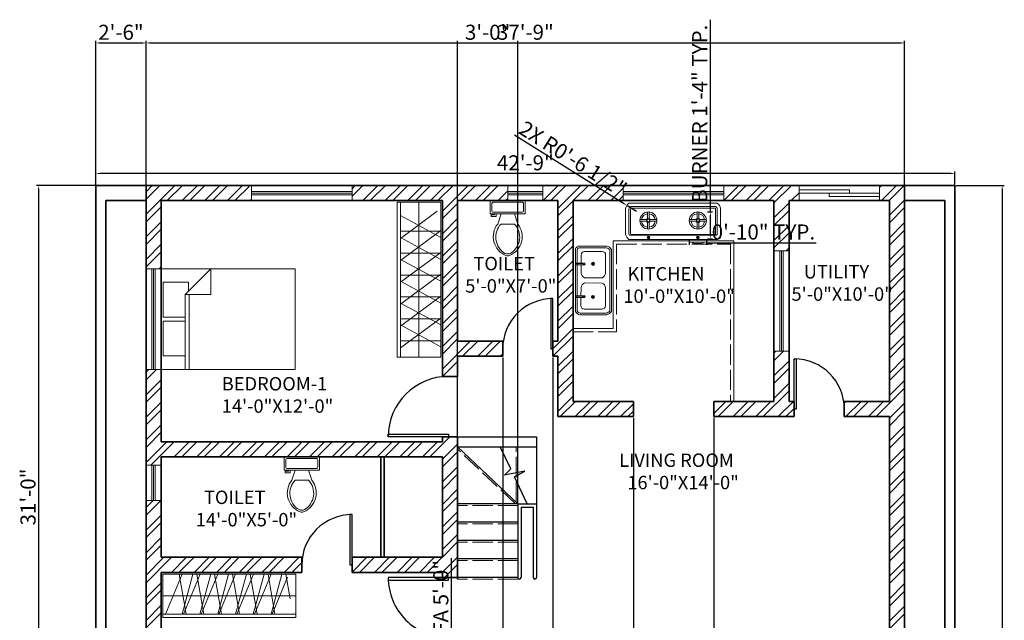
# Model space of a CAD drawing. Units: inches. Extents: x 451 to 1761, y 2292 to 3014.
# Tile 2 of 3: x 451 to 1039, y 2655 to 3014. Entities that reach past the tile are written whole.
import ezdxf

# ---------------------------------------------------------------- set-up
doc = ezdxf.new("R2010")
doc.units = ezdxf.units.IN
doc.linetypes.add('ACAD_ISO02W100', pattern=[15, 12, -3])
for name, color, linetype, lineweight in [('A-ANNO-DIMS', 2, 'Continuous', 18), ('A-AREA-IDEN', 7, 'Continuous', 18), ('A-DOOR', 4, 'Continuous', 25), ('A-EQPM', 8, 'Continuous', 18), ('A-FLOR-CASE', 9, 'Continuous', 18), ('A-FLOR-CASE-HIDN', 9, 'ACAD_ISO02W100', 13), ('A-FLOR-CASE-PATT', 252, 'Continuous', 13), ('A-FLOR-FIXT', 9, 'Continuous', 18), ('A-FLOR-STRS', 7, 'Continuous', 25), ('A-FLOR-STRS-HIDN', 8, 'ACAD_ISO02W100', 13), ('A-FURN', 8, 'Continuous', 18), ('A-GLAZ', 244, 'Continuous', 18), ('A-WALL', 7, 'Continuous', 35), ('A-WALL-PATT', 252, 'Continuous', 13), ('C-PROP', 7, 'Continuous', 35)]:
    doc.layers.add(name, color=color, linetype=linetype, lineweight=lineweight)
doc.styles.get("Standard").update_dxf_attribs({"font": 'arial.ttf'})
doc.dimstyles.new('ISO-25', dxfattribs={"dimtxt": 9, "dimasz": 2.5, "dimexe": 1.25, "dimexo": 0.625, "dimtad": 1, "dimlunit": 3, "dimtxsty": 'Standard', "dimcen": 2.5, "dimadec": 0, "dimazin": 0, "dimtfac": 1, "dimtmove": 0, "dimatfit": 3, "dimfxl": 1, "dimarcsym": 0})

# ---------------------------------------------------------------- blocks, each defined once
blk = doc.blocks.new('*D1')
at = {"layer": 'A-ANNO-DIMS', "color": 0, "lineweight": -2, "transparency": 16777216}
for p, q in [((496.79, 2915.38), (496.79, 2923.19)), ((1009.79, 2915.38), (1009.79, 2923.19)), ((1007.29, 2921.94), (499.29, 2921.94))]:
    blk.add_line(p, q, dxfattribs=at)
at = {"layer": 'A-ANNO-DIMS', "color": 0, "transparency": 16777216}
for points in [[(499.29, 2922.36), (499.29, 2921.52), (496.79, 2921.94)], [(1007.29, 2922.36), (1007.29, 2921.52), (1009.79, 2921.94)]]:
    blk.add_solid(points, dxfattribs=at)
at = {"layer": 'Defpoints', "color": 0, "transparency": 16777216}
for p in [(496.79, 2921.94), (496.79, 2914.76), (1009.79, 2914.76)]:
    blk.add_point(p, dxfattribs=at)
at = {"layer": 'A-ANNO-DIMS', "color": 0, "transparency": 16777216, "insert": (753.29, 2927.16), "char_height": 9, "attachment_point": 5}
blk.add_mtext('42\'-9"', dxfattribs=at)
blk = doc.blocks.new('*U3')
for p, q in [((0, 0), (0, 6)), ((40, 0), (40, 6))]:
    blk.add_line(p, q)
blk.add_lwpolyline([(0, 0), (0, -40), (1.75, -40), (1.75, 0)], close=True)
blk.add_arc((0, 0), 40, 270, 0)
blk = doc.blocks.new('*U4')
for p, q in [((-40, 0), (-40, 6)), ((0, 0), (0, 6))]:
    blk.add_line(p, q)
blk.add_lwpolyline([(0, 0), (0, -40), (-1.75, -40), (-1.75, 0)], close=True)
blk.add_arc((0, 0), 40, 180, 270)
blk = doc.blocks.new('*U5')
for p, q in [((0, 0), (0, 6)), ((40, 0), (40, 6))]:
    blk.add_line(p, q)
blk.add_lwpolyline([(0, 0), (0, -40), (1.75, -40), (1.75, 0)], close=True)
blk.add_arc((0, 0), 40, 270, 0)
blk = doc.blocks.new('Bed - Queen')
for p, q in [((0, -80.00003), (0, 0)), ((0, 0), (59.99999, 0)), ((59.99999, 0), (59.99999, -80.00003)), ((7.99999, -1.2), (28.79998, -1.2)), ((7.99999, -14.4), (7.99999, -1.2)), ((28.79998, -1.2), (28.79998, -14.4)), ((31.19999, -1.2), (51.99999, -1.2)), ((31.19999, -14.4), (31.19999, -1.2)), ((51.99999, -1.2), (51.99999, -16.4)), ((0, -14.4), (44.8, -14.4)), ((44.8, -16.8), (0, -16.8)), ((59.99999, -29.6), (44.8, -14.4)), ((44.8, -14.4), (44.8, -29.6)), ((51.99999, -16.4), (46.79936, -16.4)), ((44.8, -29.6), (59.99999, -29.6)), ((59.99999, -80.00003), (0, -80.00003))]:
    blk.add_line(p, q)
blk = doc.blocks.new('*U10')
for p, q in [((9.5, -6), (9.5, -2)), ((-10, -8.5), (-8, -8.5)), ((-10, -9.5), (-10, -8.5)), ((-7, -9.5), (-10, -9.5)), ((-8, -8.5), (-8, -8)), ((-7, -8), (-7, -9.5)), ((-4, -8), (-6, -14)), ((4, -8), (6, -14)), ((4, -14), (-4, -14))]:
    blk.add_line(p, q)
blk.add_lwpolyline([(10.5, -8), (10.5, 0), (-10.5, 0), (-10.5, -8)], close=True)
for points in [[(-9.5, -2), (-9.5, -6)], [(8.5, -1), (-8.5, -1)], [(-8.5, -7), (8.5, -7)]]:
    blk.add_lwpolyline(points)
for centre, radius, start, end in [((-8.62, -1.88), 0.884, 81.8699, 188.1301), ((8.62, -1.88), 0.884, 351.8699, 98.1301), ((-8.62, -6.12), 0.884, 171.8699, 278.1301), ((8.62, -6.12), 0.884, 261.8699, 8.1301), ((3.52, -21.58), 12.17, 141.46911, 247.97143), ((4.2, -21.82), 11.33, 136.36773, 238.94682), ((-3.52, -21.58), 12.17, 292.02843, 38.53071), ((-4.2, -21.82), 11.33, 301.05301, 43.63209), ((0, -27.88), 4, 245.73182, 294.26817), ((0, -29), 4, 254.86053, 285.13947)]:
    blk.add_arc(centre, radius, start, end)
blk = doc.blocks.new('*D13')
at = {"layer": 'A-ANNO-DIMS', "color": 0, "lineweight": -2, "transparency": 16777216}
for p, q in [((1010.42, 2914.76), (1039.33, 2914.76)), ((1038.08, 2912.26), (1038.08, 2332.26)), ((1010.42, 2329.76), (1039.33, 2329.76))]:
    blk.add_line(p, q, dxfattribs=at)
at = {"layer": 'A-ANNO-DIMS', "color": 0, "transparency": 16777216}
for points in [[(1037.66, 2912.26), (1038.49, 2912.26), (1038.08, 2914.76)], [(1037.66, 2332.26), (1038.49, 2332.26), (1038.08, 2329.76)]]:
    blk.add_solid(points, dxfattribs=at)
at = {"layer": 'Defpoints', "color": 0, "transparency": 16777216}
for p in [(1009.79, 2914.76), (1009.79, 2329.76), (1038.08, 2329.76)]:
    blk.add_point(p, dxfattribs=at)
at = {"layer": 'A-ANNO-DIMS', "color": 0, "transparency": 16777216, "insert": (1032.86, 2622.26), "char_height": 9, "attachment_point": 5, "rotation": 90}
blk.add_mtext('48\'-9"', dxfattribs=at)
blk = doc.blocks.new('WIN-60IN')
for p, q in [((0, 5.5), (60, 5.5)), ((0, 4.5), (60, 4.5)), ((0, 3.5), (60, 3.5))]:
    blk.add_line(p, q)
blk.add_lwpolyline([(0, 0), (0, 9), (60, 9), (60, 0)], close=True)
blk = doc.blocks.new('WIN-21IN')
for p, q in [((3.5, 0), (3.5, 21)), ((4.5, 0), (4.5, 21)), ((5.5, 0), (5.5, 21))]:
    blk.add_line(p, q)
blk.add_lwpolyline([(0, 0), (0, 21), (9, 21), (9, 0)], close=True)
blk = doc.blocks.new('COOKTOP-BURNER-AND-CONTROL')
for p, q in [((4.19, 11.76), (5.99, 11.76)), ((4.19, 11.76), (4.19, 9.96)), ((4.59, 15.93), (4.59, 11.36)), ((5.59, 15.93), (5.59, 11.36)), ((5.99, 11.76), (5.99, 9.96)), ((0.02, 11.36), (4.59, 11.36)), ((0.02, 10.36), (4.59, 10.36)), ((4.19, 9.96), (5.99, 9.96)), ((4.39, 11.56), (4.39, 10.16)), ((4.39, 11.56), (5.79, 11.56)), ((4.39, 10.16), (5.79, 10.16)), ((4.59, 10.36), (4.59, 5.79)), ((5.59, 11.36), (10.16, 11.36)), ((5.59, 10.36), (5.59, 5.79)), ((5.59, 10.36), (10.16, 10.36)), ((5.79, 11.56), (5.79, 10.16)), ((4.31, 0.88), (5.88, 0.88)), ((4.31, 0.68), (5.88, 0.68))]:
    blk.add_line(p, q)
for centre, radius in [((5.09, 10.86), 5.09), ((5.09, 0.78), 0.781)]:
    blk.add_circle(centre, radius)
for centre, radius, start, end in [((5.09, 10.86), 4.09, 97.01492, 172.98508), ((5.09, 10.86), 4.09, 7.01492, 82.98508), ((5.09, 10.86), 4.09, 187.01492, 262.98508), ((5.09, 10.86), 4.09, 277.01492, 352.98508), ((5.09, 0.78), 0.581, 9.9152, 170.0848), ((5.09, 0.78), 0.581, 189.9152, 350.0848)]:
    blk.add_arc(centre, radius, start, end)
blk = doc.blocks.new('*D30')
at = {"layer": 'A-ANNO-DIMS', "color": 0, "lineweight": -2, "transparency": 16777216}
for p, q in [((863.8, 2898.96), (863.8, 3013.76)), ((862.04, 2898.96), (865.05, 2898.96)), ((863.8, 2885.5), (863.8, 2896.46)), ((862.04, 2883), (865.05, 2883))]:
    blk.add_line(p, q, dxfattribs=at)
at = {"layer": 'A-ANNO-DIMS', "color": 0, "transparency": 16777216}
for points in [[(863.39, 2896.46), (864.22, 2896.46), (863.8, 2898.96)], [(863.39, 2885.5), (864.22, 2885.5), (863.8, 2883)]]:
    blk.add_solid(points, dxfattribs=at)
at = {"layer": 'Defpoints', "color": 0, "transparency": 16777216}
for p in [(861.41, 2898.96), (863.8, 2898.96), (861.41, 2883)]:
    blk.add_point(p, dxfattribs=at)
at = {"layer": 'A-ANNO-DIMS', "color": 0, "transparency": 16777216, "insert": (858.58, 2957.61), "char_height": 9, "attachment_point": 5, "rotation": 90}
blk.add_mtext('BURNER 1\'-4" TYP.', dxfattribs=at)
blk = doc.blocks.new('*D31')
at = {"layer": 'A-ANNO-DIMS', "color": 0, "lineweight": -2, "transparency": 16777216}
for p, q in [((851.22, 2882.38), (851.22, 2879.36)), ((861.41, 2882.38), (861.41, 2879.36)), ((853.72, 2880.61), (858.91, 2880.61)), ((861.41, 2880.61), (927.01, 2880.61))]:
    blk.add_line(p, q, dxfattribs=at)
at = {"layer": 'A-ANNO-DIMS', "color": 0, "transparency": 16777216}
for points in [[(853.72, 2881.03), (853.72, 2880.19), (851.22, 2880.61)], [(858.91, 2881.03), (858.91, 2880.19), (861.41, 2880.61)]]:
    blk.add_solid(points, dxfattribs=at)
at = {"layer": 'Defpoints', "color": 0, "transparency": 16777216}
for p in [(851.22, 2883), (861.41, 2883), (861.41, 2880.61)]:
    blk.add_point(p, dxfattribs=at)
at = {"layer": 'A-ANNO-DIMS', "color": 0, "transparency": 16777216, "insert": (895.46, 2885.83), "char_height": 9, "attachment_point": 5}
blk.add_mtext('0\'-10" TYP.', dxfattribs=at)
blk = doc.blocks.new('*D32')
at = {"layer": 'A-ANNO-DIMS', "color": 0, "lineweight": -2, "transparency": 16777216}
for p, q in [((709.28, 2626.98), (709.28, 2692.34)), ((717.66, 2626.98), (708.03, 2626.98)), ((709.28, 2569.48), (709.28, 2624.48)), ((717.66, 2566.98), (708.03, 2566.98))]:
    blk.add_line(p, q, dxfattribs=at)
at = {"layer": 'A-ANNO-DIMS', "color": 0, "transparency": 16777216}
for points in [[(708.87, 2624.48), (709.7, 2624.48), (709.28, 2626.98)], [(708.87, 2569.48), (709.7, 2569.48), (709.28, 2566.98)]]:
    blk.add_solid(points, dxfattribs=at)
at = {"layer": 'Defpoints', "color": 0, "transparency": 16777216}
for p in [(709.28, 2626.98), (718.28, 2626.98), (718.28, 2566.98)]:
    blk.add_point(p, dxfattribs=at)
at = {"layer": 'A-ANNO-DIMS', "color": 0, "transparency": 16777216, "insert": (704, 2660.91), "char_height": 9, "attachment_point": 5, "rotation": 90}
blk.add_mtext('SOFA 5\'-0"', dxfattribs=at)
blk = doc.blocks.new('*D34')
at = {"layer": 'A-ANNO-DIMS', "color": 0, "lineweight": -2, "transparency": 16777216}
for p, q in [((526.79, 2915.38), (526.79, 3001.11)), ((529.29, 2999.86), (977.29, 2999.86)), ((979.79, 2915.38), (979.79, 3001.11))]:
    blk.add_line(p, q, dxfattribs=at)
at = {"layer": 'A-ANNO-DIMS', "color": 0, "transparency": 16777216}
for points in [[(529.29, 3000.28), (529.29, 2999.44), (526.79, 2999.86)], [(977.29, 3000.28), (977.29, 2999.44), (979.79, 2999.86)]]:
    blk.add_solid(points, dxfattribs=at)
at = {"layer": 'Defpoints', "color": 0, "transparency": 16777216}
for p in [(979.79, 2999.86), (526.79, 2914.76), (979.79, 2914.76)]:
    blk.add_point(p, dxfattribs=at)
at = {"layer": 'A-ANNO-DIMS', "color": 0, "transparency": 16777216, "insert": (753.29, 3005.08), "char_height": 9, "attachment_point": 5}
blk.add_mtext('37\'-9"', dxfattribs=at)
blk = doc.blocks.new('*D35')
at = {"layer": 'A-ANNO-DIMS', "color": 0, "lineweight": -2, "transparency": 16777216}
for p, q in [((526.17, 2914.76), (461.44, 2914.76)), ((462.69, 2545.26), (462.69, 2912.26)), ((526.17, 2542.76), (461.44, 2542.76))]:
    blk.add_line(p, q, dxfattribs=at)
at = {"layer": 'A-ANNO-DIMS', "color": 0, "transparency": 16777216}
for points in [[(462.27, 2912.26), (463.11, 2912.26), (462.69, 2914.76)], [(462.27, 2545.26), (463.11, 2545.26), (462.69, 2542.76)]]:
    blk.add_solid(points, dxfattribs=at)
at = {"layer": 'Defpoints', "color": 0, "transparency": 16777216}
for p in [(462.69, 2914.76), (526.79, 2914.76), (526.79, 2542.76)]:
    blk.add_point(p, dxfattribs=at)
at = {"layer": 'A-ANNO-DIMS', "color": 0, "transparency": 16777216, "insert": (457.47, 2728.76), "char_height": 9, "attachment_point": 5, "rotation": 90}
blk.add_mtext('31\'-0"', dxfattribs=at)
blk = doc.blocks.new('*D36')
at = {"layer": 'A-ANNO-DIMS', "color": 0, "lineweight": -2, "transparency": 16777216}
for p, q in [((496.79, 2915.38), (496.79, 3001.11)), ((499.29, 2999.86), (524.29, 2999.86)), ((526.79, 2915.38), (526.79, 3001.11))]:
    blk.add_line(p, q, dxfattribs=at)
at = {"layer": 'A-ANNO-DIMS', "color": 0, "transparency": 16777216}
for points in [[(499.29, 3000.28), (499.29, 2999.44), (496.79, 2999.86)], [(524.29, 3000.28), (524.29, 2999.44), (526.79, 2999.86)]]:
    blk.add_solid(points, dxfattribs=at)
at = {"layer": 'Defpoints', "color": 0, "transparency": 16777216}
for p in [(526.79, 2999.86), (496.79, 2914.76), (526.79, 2914.76)]:
    blk.add_point(p, dxfattribs=at)
at = {"layer": 'A-ANNO-DIMS', "color": 0, "transparency": 16777216, "insert": (511.79, 3005.08), "char_height": 9, "attachment_point": 5}
blk.add_mtext('2\'-6"', dxfattribs=at)
blk = doc.blocks.new('*D38')
at = {"layer": 'A-ANNO-DIMS', "color": 0, "lineweight": -2, "transparency": 16777216}
for p, q in [((817.79, 2776.13), (817.79, 2294.1)), ((865.79, 2776.13), (865.79, 2294.1)), ((820.29, 2295.35), (863.29, 2295.35))]:
    blk.add_line(p, q, dxfattribs=at)
at = {"layer": 'A-ANNO-DIMS', "color": 0, "transparency": 16777216}
for points in [[(820.29, 2295.77), (820.29, 2294.93), (817.79, 2295.35)], [(863.29, 2295.77), (863.29, 2294.93), (865.79, 2295.35)]]:
    blk.add_solid(points, dxfattribs=at)
at = {"layer": 'Defpoints', "color": 0, "transparency": 16777216}
for p in [(817.79, 2776.76), (865.79, 2776.76), (865.79, 2295.35)]:
    blk.add_point(p, dxfattribs=at)
at = {"layer": 'A-ANNO-DIMS', "color": 0, "transparency": 16777216, "insert": (841.79, 2300.57), "char_height": 9, "attachment_point": 5}
blk.add_mtext('4\'-0"', dxfattribs=at)
blk = doc.blocks.new('*D39')
at = {"layer": 'A-ANNO-DIMS', "color": 0, "lineweight": -2, "transparency": 16777216}
for p, q in [((739.79, 2812.13), (739.79, 2294.1)), ((769.79, 2812.13), (769.79, 2294.1)), ((742.29, 2295.35), (767.29, 2295.35))]:
    blk.add_line(p, q, dxfattribs=at)
at = {"layer": 'A-ANNO-DIMS', "color": 0, "transparency": 16777216}
for points in [[(742.29, 2295.77), (742.29, 2294.93), (739.79, 2295.35)], [(767.29, 2295.77), (767.29, 2294.93), (769.79, 2295.35)]]:
    blk.add_solid(points, dxfattribs=at)
at = {"layer": 'Defpoints', "color": 0, "transparency": 16777216}
for p in [(739.79, 2812.76), (769.79, 2812.76), (769.79, 2295.35)]:
    blk.add_point(p, dxfattribs=at)
at = {"layer": 'A-ANNO-DIMS', "color": 0, "transparency": 16777216, "insert": (754.79, 2300.57), "char_height": 9, "attachment_point": 5}
blk.add_mtext('2\'-6"', dxfattribs=at)
blk = doc.blocks.new('*D40')
at = {"layer": 'A-ANNO-DIMS', "color": 0, "lineweight": -2, "transparency": 16777216}
for p, q in [((712.79, 2725.38), (712.79, 3001.11)), ((715.29, 2999.86), (746.29, 2999.86)), ((748.79, 2725.38), (748.79, 3001.11))]:
    blk.add_line(p, q, dxfattribs=at)
at = {"layer": 'A-ANNO-DIMS', "color": 0, "transparency": 16777216}
for points in [[(715.29, 3000.28), (715.29, 2999.44), (712.79, 2999.86)], [(746.29, 3000.28), (746.29, 2999.44), (748.79, 2999.86)]]:
    blk.add_solid(points, dxfattribs=at)
at = {"layer": 'Defpoints', "color": 0, "transparency": 16777216}
for p in [(748.79, 2999.86), (712.79, 2724.76), (748.79, 2724.76)]:
    blk.add_point(p, dxfattribs=at)
at = {"layer": 'A-ANNO-DIMS', "color": 0, "transparency": 16777216, "insert": (730.79, 3005.08), "char_height": 9, "attachment_point": 5}
blk.add_mtext('3\'-0"', dxfattribs=at)
blk = doc.blocks.new('*D50')
at = {"layer": 'A-ANNO-DIMS', "color": 0, "lineweight": -2, "transparency": 16777216}
for p, q in [((746.91, 2945.09), (811.85, 2904.17)), ((819.62, 2899.27), (813.96, 2902.84))]:
    blk.add_line(p, q, dxfattribs=at)
at = {"layer": 'A-ANNO-DIMS', "color": 0, "transparency": 16777216}
blk.add_solid([(812.07, 2904.52), (811.62, 2903.82), (813.96, 2902.84)], dxfattribs=at)
at = {"layer": 'Defpoints', "color": 0, "transparency": 16777216}
for p in [(813.96, 2902.84), (819.62, 2899.27)]:
    blk.add_point(p, dxfattribs=at)
at = {"layer": 'A-ANNO-DIMS', "color": 0, "transparency": 16777216, "insert": (781.14, 2929.76), "char_height": 9, "attachment_point": 5, "rotation": 327.78482}
blk.add_mtext('2X R0\'-6 1/2"', dxfattribs=at)

msp = doc.modelspace()

# ---------------------------------------------------------------- hatches: boundary and pattern name
at = {"layer": 'A-FLOR-CASE-PATT'}
h = msp.add_hatch(dxfattribs=at)
h.set_pattern_fill('ANSI31', color=256, scale=3.30105, angle=-8.34027, style=0)
h.paths.add_polyline_path([(678.791, 2812.185), (702.791, 2830.048), (702.791, 2895.374), (697.845, 2904.759), (678.791, 2890.577)])
h = msp.add_hatch(dxfattribs=at)
h.set_pattern_fill('ANSI31', color=256, scale=3.6142, angle=106.4368, style=0)
h.paths.add_polyline_path([(678.791, 2825.251), (702.791, 2812.185), (702.791, 2890.577), (678.791, 2903.642)])
h = msp.add_hatch(dxfattribs=at)
h.set_pattern_fill('ANSI31', color=256, scale=4.11503, angle=-45, style=0)
h.paths.add_polyline_path([(678.791, 2817.788), (702.791, 2817.788), (702.791, 2896.179), (678.791, 2896.179)])
h = msp.add_hatch(dxfattribs=at)
h.set_pattern_fill('ANSI31', color=256, scale=3.09097, angle=22.4971, style=0)
h.paths.add_polyline_path([(536.791, 2658.759), (611.15, 2658.759), (616.169, 2670.873), (610.47, 2682.759), (546.734, 2682.759)])
h = msp.add_hatch(dxfattribs=at)
h.set_pattern_fill('ANSI31', color=256, scale=3.29706, angle=54.7844, style=0)
h.paths.add_polyline_path([(540.402, 2682.759), (544.541, 2658.759), (608.277, 2658.759), (616.169, 2674.596), (614.761, 2682.759)])
h = msp.add_hatch(dxfattribs=at)
h.set_pattern_fill('ANSI31', color=256, scale=3.22993, angle=29.8819, style=0)
h.paths.add_polyline_path([(544.541, 2658.759), (608.277, 2658.759), (614.761, 2682.759), (551.025, 2682.759)])
at = {"layer": 'A-WALL-PATT'}
h = msp.add_hatch(dxfattribs=at)
h.set_pattern_fill('ANSI32', color=256)
h.paths.add_polyline_path([(703.791, 2551.759), (634.026, 2551.759), (634.026, 2542.759), (743.266, 2542.759), (743.266, 2551.759), (712.791, 2551.759), (712.791, 2644.759), (707.391, 2644.759), (703.791, 2644.759)])
h.paths.add_polyline_path([(535.791, 2551.759), (535.791, 2587.758), (526.791, 2587.758), (526.791, 2542.759), (574.026, 2542.759), (574.026, 2551.759)])
h.paths.add_polyline_path([(526.791, 2647.758), (535.791, 2647.758), (535.791, 2683.759), (619.791, 2683.759), (619.791, 2692.759), (535.791, 2692.759), (535.791, 2726.772), (526.791, 2726.772)])
h.paths.add_polyline_path([(649.791, 2692.759), (649.791, 2683.759), (703.791, 2683.759), (703.791, 2680.759), (712.791, 2680.759), (712.791, 2752.759), (712.791, 2764.759), (703.791, 2764.759), (703.791, 2761.759), (535.791, 2761.759), (535.791, 2804.959), (526.791, 2804.959), (526.791, 2747.772), (535.791, 2747.772), (535.791, 2752.759), (703.791, 2752.759), (703.791, 2692.759)])
h.paths.add_polyline_path([(781.791, 2785.759), (781.791, 2905.759), (811.791, 2905.759), (811.791, 2914.759), (763.791, 2914.759), (763.791, 2905.759), (772.791, 2905.759), (772.791, 2821.759), (769.791, 2821.759), (769.791, 2812.759), (772.791, 2812.759), (772.791, 2776.759), (817.791, 2776.759), (817.791, 2785.759)])
h.paths.add_polyline_path([(703.791, 2800.759), (712.791, 2800.759), (712.791, 2812.759), (739.791, 2812.759), (739.791, 2821.759), (712.791, 2821.759), (712.791, 2905.759), (742.791, 2905.759), (742.791, 2914.759), (649.791, 2914.759), (649.791, 2905.759), (703.791, 2905.759)])
h.paths.add_polyline_path([(526.791, 2864.959), (535.791, 2864.959), (535.791, 2905.759), (589.791, 2905.759), (589.791, 2914.759), (526.791, 2914.759)])
h.paths.add_polyline_path([(901.791, 2905.759), (901.791, 2875.759), (910.791, 2875.759), (910.791, 2905.759), (916.791, 2905.759), (916.791, 2914.759), (871.791, 2914.759), (871.791, 2905.759)])
h.paths.add_polyline_path([(901.791, 2785.759), (865.791, 2785.759), (865.791, 2776.759), (901.791, 2776.759), (913.791, 2776.759), (913.791, 2781.259), (913.791, 2785.759), (910.791, 2785.759), (910.791, 2815.759), (901.791, 2815.759)])
h.paths.add_polyline_path([(979.791, 2914.759), (964.791, 2914.759), (964.791, 2905.759), (970.791, 2905.759), (970.791, 2785.759), (943.791, 2785.759), (943.791, 2776.759), (970.791, 2776.759), (970.791, 2551.759), (961.316, 2551.759), (961.316, 2542.759), (979.791, 2542.759)])
h.paths.add_polyline_path([(901.316, 2542.759), (901.316, 2551.759), (889.791, 2551.759), (889.791, 2647.758), (880.791, 2647.758), (880.791, 2551.759), (877.791, 2551.759), (877.791, 2542.759)])
h.paths.add_polyline_path([(803.266, 2551.759), (803.266, 2542.759), (829.791, 2542.759), (829.791, 2551.759)])

# ---------------------------------------------------------------- linework, layer by layer
at = {"layer": 'A-EQPM'}
for points in [[(813.189, 2901.108, -0.1431126), (815.189, 2904.282), (867.926, 2904.282, -0.1431126), (869.926, 2901.108), (869.926, 2885.578, -0.1653839), (867.926, 2882.553), (815.189, 2882.553, -0.1653839), (813.189, 2885.578)], [(815.189, 2900.803, -0.0913821), (816.025, 2902.282), (867.089, 2902.282, -0.0913821), (867.926, 2900.803), (867.926, 2885.864, -0.4371352), (867.156, 2885.017), (815.958, 2885.017, -0.4371352), (815.189, 2885.864)], [(816.189, 2900.625, -0.0502493), (816.527, 2901.282), (866.587, 2901.282, -0.0502493), (866.926, 2900.625), (866.926, 2886.039, -0.0522238), (866.672, 2885.553), (816.442, 2885.553, -0.0522238), (816.189, 2886.039)]]:
    msp.add_lwpolyline(points, format="xyb", close=True, dxfattribs=at)
at = {"layer": 'A-FLOR-CASE'}
for p, q in [((676.791, 2904.759), (702.791, 2904.759)), ((676.791, 2904.759), (676.791, 2812.185)), ((678.791, 2904.759), (678.791, 2812.185)), ((689.791, 2904.759), (689.791, 2812.185)), ((702.791, 2904.759), (702.791, 2812.185)), ((805.791, 2881.759), (877.791, 2881.759)), ((805.791, 2881.759), (805.791, 2829.446)), ((877.791, 2881.759), (877.791, 2785.759)), ((781.791, 2829.446), (805.791, 2829.446)), ((702.791, 2812.185), (676.791, 2812.185)), ((536.791, 2682.759), (616.169, 2682.759)), ((536.791, 2682.759), (536.791, 2656.759)), ((616.169, 2682.759), (616.169, 2656.759)), ((536.791, 2669.759), (616.169, 2669.759)), ((536.791, 2658.759), (616.169, 2658.759)), ((536.791, 2656.759), (616.169, 2656.759))]:
    msp.add_line(p, q, dxfattribs=at)
at = {"layer": 'A-FLOR-CASE-HIDN'}
for p, q in [((807.791, 2879.759), (807.791, 2827.446)), ((807.791, 2879.759), (875.791, 2879.759)), ((875.791, 2879.759), (875.791, 2785.759)), ((781.791, 2827.446), (807.791, 2827.446))]:
    msp.add_line(p, q, dxfattribs=at)
at = {"layer": 'A-FLOR-FIXT'}
for p, q in [((788.042, 2868.362), (783.226, 2868.362)), ((787.944, 2868.262), (783.226, 2868.262)), ((787.976, 2867.462), (783.226, 2867.462)), ((788.094, 2867.362), (783.226, 2867.362)), ((788.45, 2867.362), (788.432, 2867.362)), ((793.014, 2867.982), (794.421, 2867.982)), ((793.199, 2868.456), (794.237, 2867.507)), ((794.231, 2868.463), (793.204, 2867.501)), ((793.718, 2868.685), (793.718, 2867.278)), ((787.947, 2847.93), (783.13, 2847.975)), ((787.849, 2848.031), (783.131, 2848.075)), ((787.889, 2848.83), (783.138, 2848.875)), ((788.008, 2848.929), (783.139, 2848.975)), ((788.363, 2848.926), (788.345, 2848.926)), ((792.922, 2848.264), (794.329, 2848.251)), ((793.102, 2847.787), (794.149, 2848.727)), ((794.134, 2847.772), (793.116, 2848.743)), ((793.619, 2847.554), (793.632, 2848.961))]:
    msp.add_line(p, q, dxfattribs=at)
for points in [[(783.226, 2876.579, -0.4142136), (785.902, 2878.579), (801.902, 2878.579, -0.2057988), (804.693, 2876.579), (804.693, 2839.566, -0.2057988), (801.902, 2837.566), (785.902, 2837.566, -0.2285234), (783.226, 2839.566)], [(784.226, 2876.497, -0.4142136), (785.82, 2877.579), (801.786, 2877.579, -0.1776882), (803.693, 2876.281), (803.693, 2839.864, -0.1776882), (801.786, 2838.566), (786.006, 2838.566, -0.1994318), (784.226, 2839.83)]]:
    msp.add_lwpolyline(points, format="xyb", close=True, dxfattribs=at)
for points in [[(786.605, 2868.362), (786.605, 2873.295, -0.4142136), (788.605, 2875.295), (799.263, 2875.295, -0.4142136), (801.263, 2873.295), (801.263, 2862.43, -0.2828706), (799.263, 2859.713), (788.605, 2859.713, -0.2828706), (786.605, 2862.43), (786.605, 2867.362)], [(786.509, 2847.943), (786.463, 2843.011, 0.4142136), (788.444, 2840.993), (799.102, 2840.893, 0.4142136), (801.12, 2842.874), (801.222, 2853.738, 0.2828706), (799.248, 2856.474), (788.59, 2856.574, 0.2828706), (786.565, 2853.875), (786.518, 2848.943)]]:
    msp.add_lwpolyline(points, format="xyb", dxfattribs=at)
for centre, radius in [((788.432, 2867.881), 0.619), ((788.432, 2867.881), 0.519), ((793.718, 2867.982), 0.903), ((793.718, 2867.982), 0.703), ((788.341, 2848.407), 0.619), ((788.341, 2848.407), 0.519), ((793.625, 2848.257), 0.903), ((793.625, 2848.257), 0.703)]:
    msp.add_circle(centre, radius, dxfattribs=at)
at = {"layer": 'A-FLOR-STRS'}
for p, q in [((712.791, 2764.759), (759.991, 2764.759)), ((759.991, 2764.759), (759.991, 2680.759)), ((712.791, 2758.759), (759.991, 2758.759)), ((748.791, 2724.759), (712.791, 2758.759)), ((748.791, 2724.759), (748.791, 2758.759)), ((748.791, 2724.759), (712.791, 2724.759)), ((748.791, 2724.759), (748.791, 2680.759)), ((748.791, 2724.759), (759.991, 2724.759)), ((750.791, 2722.759), (750.791, 2680.759)), ((750.791, 2722.759), (757.991, 2722.759)), ((757.991, 2722.759), (757.991, 2680.759)), ((748.791, 2713.759), (712.791, 2713.759)), ((748.791, 2702.759), (712.791, 2702.759)), ((748.791, 2691.759), (712.791, 2691.759)), ((748.791, 2680.759), (712.791, 2680.759)), ((748.791, 2680.759), (748.791, 2679.759))]:
    msp.add_line(p, q, dxfattribs=at)
msp.add_lwpolyline([(754.391, 2724.759), (746.777, 2740.905), (753.023, 2744.188), (740.893, 2741.725), (744.57, 2745.584), (738.357, 2758.759)], dxfattribs=at)
for centre in [(749.791, 2680.776), (758.991, 2680.776)]:
    msp.add_arc(centre, 1, 181.02435, 358.97565, dxfattribs=at)
at = {"layer": 'A-FLOR-STRS-HIDN'}
for p, q in [((747.791, 2725.703), (747.791, 2758.759)), ((747.335, 2724.759), (712.791, 2757.383)), ((748.791, 2723.759), (712.791, 2723.759)), ((748.791, 2712.759), (712.791, 2712.759)), ((748.791, 2701.759), (712.791, 2701.759)), ((748.791, 2690.759), (712.791, 2690.759)), ((748.791, 2679.759), (712.791, 2679.759))]:
    msp.add_line(p, q, dxfattribs=at)
at = {"layer": 'A-GLAZ'}
for p, q in [((916.791, 2905.759), (916.791, 2914.759)), ((916.791, 2912.259), (946.791, 2912.259)), ((946.791, 2910.259), (946.791, 2912.259)), ((964.791, 2905.759), (964.791, 2914.759)), ((916.791, 2910.259), (964.791, 2910.259)), ((934.791, 2908.259), (934.791, 2910.259)), ((934.791, 2908.259), (964.791, 2908.259))]:
    msp.add_line(p, q, dxfattribs=at)
at = {"layer": 'A-WALL'}
for p, q in [((526.791, 2914.759), (526.791, 2542.759)), ((979.791, 2914.759), (979.791, 2542.759)), ((535.791, 2905.759), (535.791, 2761.759)), ((535.791, 2905.759), (703.791, 2905.759)), ((703.791, 2905.759), (703.791, 2800.759)), ((712.791, 2905.759), (712.791, 2821.759)), ((712.791, 2905.759), (772.791, 2905.759)), ((772.791, 2905.759), (772.791, 2821.759)), ((781.791, 2905.759), (781.791, 2785.759)), ((781.791, 2905.759), (901.791, 2905.759)), ((901.791, 2905.759), (901.791, 2785.759)), ((910.791, 2905.759), (910.791, 2785.759)), ((910.791, 2905.759), (970.791, 2905.759)), ((970.791, 2905.759), (970.791, 2785.759)), ((712.791, 2821.759), (739.791, 2821.759)), ((739.791, 2821.759), (739.791, 2812.759)), ((769.791, 2821.759), (769.791, 2812.759)), ((769.791, 2821.759), (772.791, 2821.759)), ((712.791, 2812.759), (739.791, 2812.759)), ((712.791, 2812.759), (712.791, 2800.759)), ((769.791, 2812.759), (772.791, 2812.759)), ((772.791, 2812.759), (772.791, 2776.759)), ((703.791, 2800.759), (712.791, 2800.759)), ((781.791, 2785.759), (817.791, 2785.759)), ((817.791, 2785.759), (817.791, 2776.759)), ((865.791, 2785.759), (865.791, 2776.759)), ((865.791, 2785.759), (901.791, 2785.759)), ((910.791, 2785.759), (913.791, 2785.759)), ((913.791, 2785.759), (913.791, 2776.759)), ((943.791, 2785.759), (943.791, 2776.759)), ((943.791, 2785.759), (970.791, 2785.759)), ((772.791, 2776.759), (817.791, 2776.759)), ((865.791, 2776.759), (901.791, 2776.759)), ((901.791, 2776.759), (913.791, 2776.759)), ((943.791, 2776.759), (970.791, 2776.759)), ((970.791, 2776.759), (970.791, 2551.759)), ((703.791, 2764.759), (712.791, 2764.759)), ((703.791, 2764.759), (703.791, 2761.759)), ((712.791, 2764.759), (712.791, 2752.759)), ((535.791, 2761.759), (703.791, 2761.759)), ((535.791, 2752.759), (535.791, 2692.759)), ((535.791, 2752.759), (703.791, 2752.759)), ((667.061, 2692.759), (667.061, 2752.759)), ((669.061, 2692.759), (669.061, 2752.759)), ((703.791, 2752.759), (703.791, 2692.759)), ((712.791, 2752.759), (712.791, 2679.759)), ((535.791, 2692.759), (619.791, 2692.759)), ((619.791, 2692.759), (619.791, 2683.759)), ((649.791, 2692.759), (649.791, 2683.759)), ((649.791, 2692.759), (703.791, 2692.759)), ((535.791, 2683.759), (619.791, 2683.759)), ((535.791, 2683.759), (535.791, 2551.759)), ((649.791, 2683.759), (703.791, 2683.759)), ((703.791, 2683.759), (703.791, 2680.759)), ((703.791, 2680.759), (712.791, 2680.759))]:
    msp.add_line(p, q, dxfattribs=at)
at = {"layer": 'C-PROP'}
for p, q in [((496.791, 2914.759), (1009.791, 2914.759)), ((496.791, 2914.759), (496.791, 2329.759)), ((1009.791, 2914.759), (1009.791, 2329.759)), ((502.791, 2905.759), (526.791, 2905.759)), ((502.791, 2905.759), (502.791, 2329.759)), ((979.791, 2905.759), (1003.791, 2905.759)), ((1003.791, 2905.759), (1003.791, 2338.759))]:
    msp.add_line(p, q, dxfattribs=at)

# ---------------------------------------------------------------- block references
at = {"layer": 'A-DOOR'}
for name, p, xscale, yscale, zscale, rotation in [('*U5', (769.791, 2817.259), 0.7499999999999943, 0.7499999999999943, 0.7499999999999943, 180), ('*U4', (913.791, 2781.259), 0.7499999999999943, 0.7499999999999943, 0.7499999999999943, 180), ('*U4', (707.391, 2764.759), 0.9000000000000111, 0.9000000000000111, 0.9000000000000111, 270), ('*U5', (649.791, 2688.259), 0.7499999999999943, 0.7499999999999943, 0.7499999999999943, 180), ('*U3', (707.391, 2680.759), 0.9000000000000111, 0.9000000000000111, 0.9000000000000111, 270)]:
    msp.add_blockref(name, p, dxfattribs=dict(at, xscale=xscale, yscale=yscale, zscale=zscale, rotation=rotation))
at = {"layer": 'A-EQPM'}
for p in [(821.704, 2883.004), (851.222, 2883.004)]:
    msp.add_blockref('COOKTOP-BURNER-AND-CONTROL', p, dxfattribs=at)
at = {"layer": 'A-FLOR-FIXT'}
for p in [(742.791, 2905.759), (619.791, 2752.759)]:
    msp.add_blockref('*U10', p, dxfattribs=at)
at = {"layer": 'A-FURN', "rotation": 90}
msp.add_blockref('Bed - Queen', (535.791, 2804.959), dxfattribs=at)
at = {"layer": 'A-GLAZ'}
for name, p in [('WIN-60IN', (589.791, 2905.759)), ('WIN-60IN', (811.791, 2905.759)), ('WIN-21IN', (526.791, 2726.772))]:
    msp.add_blockref(name, p, dxfattribs=at)
for name, p, rotation in [('WIN-21IN', (742.791, 2914.759), 269.9999999999987), ('WIN-60IN', (901.792, 2875.759), 269.9999999999998), ('WIN-60IN', (526.792, 2864.959), 269.9999999999997)]:
    msp.add_blockref(name, p, dxfattribs=dict(at, rotation=rotation))

# ---------------------------------------------------------------- texts
at = {"layer": 'A-AREA-IDEN', "char_height": 8, "attachment_point": 1}
for s, width, insert in [('  TOILET \\P5\'-0"X7\'-0"', 52.38915, (717.389, 2872.137)), (' KITCHEN\\P10\'-0"X10\'-0"', 64.48945, (811.828, 2866.006)), ('   UTILITY\\P5\'-0"X10\'-0"', 58.56076, (912.23, 2867.261)), ('BEDROOM-1 \\P14\'-0"X12\'-0"', 67.82233, (572.018, 2800.37)), ('LIVING ROOM \\P  16\'-0"X14\'-0"', 75.6515, (809.31, 2754.736)), ('  TOILET \\P14\'-0"X5\'-0"', 52.38915, (556.489, 2732.571))]:
    msp.add_mtext_dynamic_manual_height_columns(s, width=width, gutter_width=12.5, heights=[0], dxfattribs=dict(at, insert=insert))

# ---------------------------------------------------------------- dimensions: what is measured, and where the dimension line sits
at = {"layer": 'A-ANNO-DIMS'}
for base, p1, p2, override, picture, middle in [((526.791, 2999.859), (496.791, 2914.759), (526.791, 2914.759), {"dimdec": 1, "dimlfac": 1, "dimrnd": 0, "dimzin": 1, "dimdsep": 46, "dimlunit": 4, "dimfrac": 2}, '*D36', (511.791, 3005.079)), ((979.791, 2999.859), (526.791, 2914.759), (979.791, 2914.759), {"dimdec": 1, "dimlfac": 1, "dimrnd": 0, "dimzin": 1, "dimdsep": 46, "dimlunit": 4, "dimfrac": 2}, '*D34', (753.291, 3005.082)), ((748.791, 2999.859), (712.791, 2724.759), (748.791, 2724.759), {"dimdec": 1, "dimlfac": 1, "dimrnd": 0, "dimzin": 1, "dimdsep": 46, "dimlunit": 4, "dimfrac": 2}, '*D40', (730.791, 3005.082)), ((496.791, 2921.94), (1009.791, 2914.759), (496.791, 2914.759), {"dimclrd": 0, "dimclre": 0, "dimclrt": 0}, '*D1', (753.291, 2927.16)), ((769.791, 2295.35), (739.791, 2812.759), (769.791, 2812.759), {"dimdec": 1, "dimlfac": 1, "dimrnd": 0, "dimzin": 1, "dimdsep": 46, "dimlunit": 4, "dimfrac": 2}, '*D39', (754.791, 2300.57)), ((865.791, 2295.35), (817.791, 2776.759), (865.791, 2776.759), {"dimdec": 1, "dimlfac": 1, "dimrnd": 0, "dimzin": 1, "dimdsep": 46, "dimlunit": 4, "dimfrac": 2}, '*D38', (841.791, 2300.57))]:
    dim = msp.add_linear_dim(base=base, p1=p1, p2=p2, dimstyle='ISO-25', override=override, dxfattribs=at)
    dim.commit()
    dim.dimension.update_dxf_attribs({"geometry": picture, "text_midpoint": middle})
for base, p1, p2, text, picture, middle in [((863.804, 2898.96), (861.41, 2883.004), (861.41, 2898.96), 'BURNER <> TYP.', '*D30', (858.584, 2957.608)), ((709.284, 2626.983), (718.284, 2566.983), (718.284, 2626.983), 'SOFA <>', '*D32', (704.002, 2660.911))]:
    dim = msp.add_linear_dim(base=base, p1=p1, p2=p2, angle=90, text=text, dimstyle='ISO-25', override={"dimdec": 1, "dimlfac": 1, "dimrnd": 0, "dimzin": 1, "dimdsep": 46, "dimlunit": 4, "dimfrac": 2}, dxfattribs=at)
    dim.commit()
    dim.dimension.update_dxf_attribs({"geometry": picture, "text_midpoint": middle})
dim = msp.add_radius_dim(center=(819.62, 2899.273), mpoint=(813.962, 2902.838), text='2X <>', dimstyle='ISO-25', override={"dimdec": 1, "dimlfac": 1, "dimrnd": 0, "dimzin": 1, "dimdsep": 46, "dimlunit": 4, "dimfrac": 2}, dxfattribs=at)
dim.commit()
dim.dimension.update_dxf_attribs({"geometry": '*D50', "text_midpoint": (781.135, 2929.761)})
for base, p1, p2, override, picture, middle in [((462.691, 2914.759), (526.791, 2542.759), (526.791, 2914.759), {"dimdec": 1, "dimlfac": 1, "dimrnd": 0, "dimzin": 1, "dimdsep": 46, "dimlunit": 4, "dimfrac": 2}, '*D35', (457.468, 2728.759)), ((1038.076, 2329.759), (1009.791, 2914.759), (1009.791, 2329.759), {"dimclrd": 0, "dimclre": 0, "dimclrt": 0}, '*D13', (1032.856, 2622.259))]:
    dim = msp.add_linear_dim(base=base, p1=p1, p2=p2, angle=90, dimstyle='ISO-25', override=override, dxfattribs=at)
    dim.commit()
    dim.dimension.update_dxf_attribs({"geometry": picture, "text_midpoint": middle})
dim = msp.add_linear_dim(base=(861.41, 2880.611), p1=(851.222, 2883.004), p2=(861.41, 2883.004), text='<> TYP.', dimstyle='ISO-25', override={"dimdec": 1, "dimlfac": 1, "dimrnd": 0, "dimzin": 1, "dimdsep": 46, "dimlunit": 4, "dimfrac": 2}, dxfattribs=at)
dim.commit()
dim.dimension.update_dxf_attribs({"geometry": '*D31', "text_midpoint": (895.461, 2885.831)})

doc.saveas('drawing.dxf')
